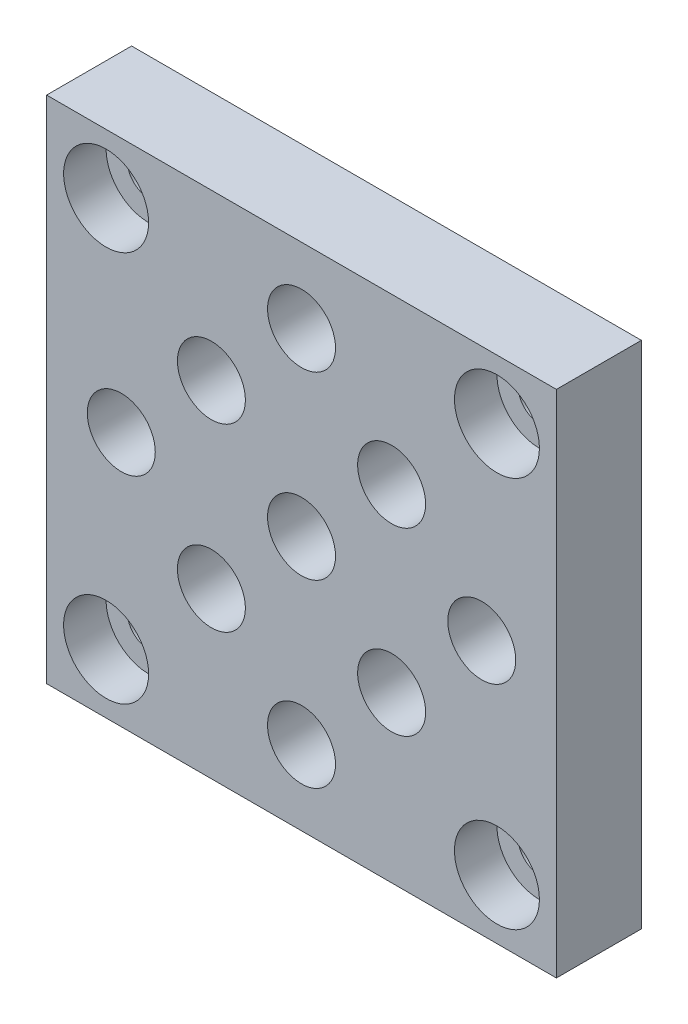
ISO-10303-21;
HEADER;
FILE_DESCRIPTION(('STEP AP214'),'2;1');
FILE_NAME('part.step','',(''),(''),'','','');
FILE_SCHEMA(('AUTOMOTIVE_DESIGN { 1 0 10303 214 1 1 1 1 }'));
ENDSEC;
DATA;
#1=APPLICATION_CONTEXT('core data for automotive mechanical design processes');
#2=APPLICATION_PROTOCOL_DEFINITION('international standard','automotive_design',2000,#1);
#3=PRODUCT_CONTEXT('',#1,'mechanical');
#4=PRODUCT('Part','Part','',(#3));
#5=PRODUCT_RELATED_PRODUCT_CATEGORY('part','',(#4));
#6=PRODUCT_DEFINITION_FORMATION('','',#4);
#7=PRODUCT_DEFINITION_CONTEXT('part definition',#1,'design');
#8=PRODUCT_DEFINITION('design','',#6,#7);
#9=PRODUCT_DEFINITION_SHAPE('','',#8);
#10=(LENGTH_UNIT() NAMED_UNIT(*) SI_UNIT(.MILLI.,.METRE.));
#11=(NAMED_UNIT(*) PLANE_ANGLE_UNIT() SI_UNIT($,.RADIAN.));
#12=(NAMED_UNIT(*) SI_UNIT($,.STERADIAN.) SOLID_ANGLE_UNIT());
#13=UNCERTAINTY_MEASURE_WITH_UNIT(LENGTH_MEASURE(1.E-05),#10,'distance_accuracy_value','');
#14=(GEOMETRIC_REPRESENTATION_CONTEXT(3) GLOBAL_UNCERTAINTY_ASSIGNED_CONTEXT((#13)) GLOBAL_UNIT_ASSIGNED_CONTEXT((#10,
#11,#12)) REPRESENTATION_CONTEXT('',''));
#15=CARTESIAN_POINT('',(0.,0.,0.));
#16=DIRECTION('',(0.,0.,1.));
#17=DIRECTION('',(1.,0.,0.));
#18=AXIS2_PLACEMENT_3D('',#15,#16,#17);
#19=CARTESIAN_POINT('',(0.,60.,10.));
#20=DIRECTION('',(1.,0.,0.));
#21=DIRECTION('',(0.,0.,-1.));
#22=AXIS2_PLACEMENT_3D('',#19,#20,#21);
#23=PLANE('',#22);
#24=DIRECTION('',(0.,-1.,0.));
#25=VECTOR('',#24,1.);
#26=CARTESIAN_POINT('',(0.,60.,0.));
#27=LINE('',#26,#25);
#28=CARTESIAN_POINT('',(0.,60.,0.));
#29=VERTEX_POINT('',#28);
#30=CARTESIAN_POINT('',(0.,0.,0.));
#31=VERTEX_POINT('',#30);
#32=EDGE_CURVE('E117',#29,#31,#27,.T.);
#33=ORIENTED_EDGE('',*,*,#32,.T.);
#34=DIRECTION('',(0.,0.,-1.));
#35=VECTOR('',#34,1.);
#36=CARTESIAN_POINT('',(0.,0.,10.));
#37=LINE('',#36,#35);
#38=CARTESIAN_POINT('',(0.,0.,10.));
#39=VERTEX_POINT('',#38);
#40=EDGE_CURVE('E12',#39,#31,#37,.T.);
#41=ORIENTED_EDGE('',*,*,#40,.F.);
#42=DIRECTION('',(0.,-1.,0.));
#43=VECTOR('',#42,1.);
#44=CARTESIAN_POINT('',(0.,60.,10.));
#45=LINE('',#44,#43);
#46=CARTESIAN_POINT('',(0.,60.,10.));
#47=VERTEX_POINT('',#46);
#48=EDGE_CURVE('E106',#47,#39,#45,.T.);
#49=ORIENTED_EDGE('',*,*,#48,.F.);
#50=DIRECTION('',(0.,0.,-1.));
#51=VECTOR('',#50,1.);
#52=CARTESIAN_POINT('',(0.,60.,10.));
#53=LINE('',#52,#51);
#54=EDGE_CURVE('E111',#47,#29,#53,.T.);
#55=ORIENTED_EDGE('',*,*,#54,.T.);
#56=EDGE_LOOP('',(#33,#41,#49,#55));
#57=FACE_BOUND('',#56,.T.);
#58=ADVANCED_FACE('F54',(#57),#23,.F.);
#59=CARTESIAN_POINT('',(0.,0.,10.));
#60=DIRECTION('',(0.,1.,0.));
#61=DIRECTION('',(0.,0.,1.));
#62=AXIS2_PLACEMENT_3D('',#59,#60,#61);
#63=PLANE('',#62);
#64=DIRECTION('',(1.,0.,0.));
#65=VECTOR('',#64,1.);
#66=CARTESIAN_POINT('',(0.,0.,0.));
#67=LINE('',#66,#65);
#68=CARTESIAN_POINT('',(60.,0.,0.));
#69=VERTEX_POINT('',#68);
#70=EDGE_CURVE('E109',#31,#69,#67,.T.);
#71=ORIENTED_EDGE('',*,*,#70,.T.);
#72=DIRECTION('',(0.,0.,-1.));
#73=VECTOR('',#72,1.);
#74=CARTESIAN_POINT('',(60.,0.,10.));
#75=LINE('',#74,#73);
#76=CARTESIAN_POINT('',(60.,0.,10.));
#77=VERTEX_POINT('',#76);
#78=EDGE_CURVE('E62',#77,#69,#75,.T.);
#79=ORIENTED_EDGE('',*,*,#78,.F.);
#80=DIRECTION('',(1.,0.,0.));
#81=VECTOR('',#80,1.);
#82=CARTESIAN_POINT('',(0.,0.,10.));
#83=LINE('',#82,#81);
#84=EDGE_CURVE('E101',#39,#77,#83,.T.);
#85=ORIENTED_EDGE('',*,*,#84,.F.);
#86=ORIENTED_EDGE('',*,*,#40,.T.);
#87=EDGE_LOOP('',(#71,#79,#85,#86));
#88=FACE_BOUND('',#87,.T.);
#89=ADVANCED_FACE('F108',(#88),#63,.F.);
#90=CARTESIAN_POINT('',(60.,0.,10.));
#91=DIRECTION('',(-1.,0.,0.));
#92=DIRECTION('',(0.,0.,1.));
#93=AXIS2_PLACEMENT_3D('',#90,#91,#92);
#94=PLANE('',#93);
#95=DIRECTION('',(0.,1.,0.));
#96=VECTOR('',#95,1.);
#97=CARTESIAN_POINT('',(60.,0.,0.));
#98=LINE('',#97,#96);
#99=CARTESIAN_POINT('',(60.,60.,0.));
#100=VERTEX_POINT('',#99);
#101=EDGE_CURVE('E86',#69,#100,#98,.T.);
#102=ORIENTED_EDGE('',*,*,#101,.T.);
#103=DIRECTION('',(0.,0.,-1.));
#104=VECTOR('',#103,1.);
#105=CARTESIAN_POINT('',(60.,60.,10.));
#106=LINE('',#105,#104);
#107=CARTESIAN_POINT('',(60.,60.,10.));
#108=VERTEX_POINT('',#107);
#109=EDGE_CURVE('E112',#108,#100,#106,.T.);
#110=ORIENTED_EDGE('',*,*,#109,.F.);
#111=DIRECTION('',(0.,1.,0.));
#112=VECTOR('',#111,1.);
#113=CARTESIAN_POINT('',(60.,0.,10.));
#114=LINE('',#113,#112);
#115=EDGE_CURVE('E102',#77,#108,#114,.T.);
#116=ORIENTED_EDGE('',*,*,#115,.F.);
#117=ORIENTED_EDGE('',*,*,#78,.T.);
#118=EDGE_LOOP('',(#102,#110,#116,#117));
#119=FACE_BOUND('',#118,.T.);
#120=ADVANCED_FACE('F115',(#119),#94,.F.);
#121=CARTESIAN_POINT('',(60.,60.,10.));
#122=DIRECTION('',(0.,-1.,0.));
#123=DIRECTION('',(0.,0.,-1.));
#124=AXIS2_PLACEMENT_3D('',#121,#122,#123);
#125=PLANE('',#124);
#126=DIRECTION('',(-1.,0.,0.));
#127=VECTOR('',#126,1.);
#128=CARTESIAN_POINT('',(60.,60.,0.));
#129=LINE('',#128,#127);
#130=EDGE_CURVE('E94',#100,#29,#129,.T.);
#131=ORIENTED_EDGE('',*,*,#130,.T.);
#132=ORIENTED_EDGE('',*,*,#54,.F.);
#133=DIRECTION('',(-1.,0.,0.));
#134=VECTOR('',#133,1.);
#135=CARTESIAN_POINT('',(60.,60.,10.));
#136=LINE('',#135,#134);
#137=EDGE_CURVE('E72',#108,#47,#136,.T.);
#138=ORIENTED_EDGE('',*,*,#137,.F.);
#139=ORIENTED_EDGE('',*,*,#109,.T.);
#140=EDGE_LOOP('',(#131,#132,#138,#139));
#141=FACE_BOUND('',#140,.T.);
#142=ADVANCED_FACE('F127',(#141),#125,.F.);
#143=CARTESIAN_POINT('',(0.,0.,10.));
#144=DIRECTION('',(0.,0.,1.));
#145=DIRECTION('',(1.,0.,0.));
#146=AXIS2_PLACEMENT_3D('',#143,#144,#145);
#147=PLANE('',#146);
#148=CARTESIAN_POINT('',(30.,51.2132034355964,10.));
#149=DIRECTION('',(0.,0.,1.));
#150=DIRECTION('',(1.,0.,0.));
#151=AXIS2_PLACEMENT_3D('',#148,#149,#150);
#152=CIRCLE('',#151,3.99999999999999);
#153=CARTESIAN_POINT('',(34.,51.2132034355964,10.));
#154=VERTEX_POINT('',#153);
#155=EDGE_CURVE('E181',#154,#154,#152,.T.);
#156=ORIENTED_EDGE('',*,*,#155,.F.);
#157=EDGE_LOOP('',(#156));
#158=FACE_BOUND('',#157,.T.);
#159=CARTESIAN_POINT('',(40.6066017177982,40.6066017177982,10.));
#160=DIRECTION('',(0.,0.,1.));
#161=DIRECTION('',(1.,0.,0.));
#162=AXIS2_PLACEMENT_3D('',#159,#160,#161);
#163=CIRCLE('',#162,4.);
#164=CARTESIAN_POINT('',(44.6066017177982,40.6066017177982,10.));
#165=VERTEX_POINT('',#164);
#166=EDGE_CURVE('E205',#165,#165,#163,.T.);
#167=ORIENTED_EDGE('',*,*,#166,.F.);
#168=EDGE_LOOP('',(#167));
#169=FACE_BOUND('',#168,.T.);
#170=CARTESIAN_POINT('',(51.2132034355964,30.,10.));
#171=DIRECTION('',(0.,0.,1.));
#172=DIRECTION('',(1.,0.,0.));
#173=AXIS2_PLACEMENT_3D('',#170,#171,#172);
#174=CIRCLE('',#173,4.);
#175=CARTESIAN_POINT('',(55.2132034355964,30.,10.));
#176=VERTEX_POINT('',#175);
#177=EDGE_CURVE('E198',#176,#176,#174,.T.);
#178=ORIENTED_EDGE('',*,*,#177,.F.);
#179=EDGE_LOOP('',(#178));
#180=FACE_BOUND('',#179,.T.);
#181=CARTESIAN_POINT('',(40.6066017177982,19.3933982822018,10.));
#182=DIRECTION('',(0.,0.,1.));
#183=DIRECTION('',(1.,0.,0.));
#184=AXIS2_PLACEMENT_3D('',#181,#182,#183);
#185=CIRCLE('',#184,4.);
#186=CARTESIAN_POINT('',(44.6066017177982,19.3933982822018,10.));
#187=VERTEX_POINT('',#186);
#188=EDGE_CURVE('E188',#187,#187,#185,.T.);
#189=ORIENTED_EDGE('',*,*,#188,.F.);
#190=EDGE_LOOP('',(#189));
#191=FACE_BOUND('',#190,.T.);
#192=CARTESIAN_POINT('',(8.78679656440358,30.,10.));
#193=DIRECTION('',(0.,0.,1.));
#194=DIRECTION('',(1.,0.,0.));
#195=AXIS2_PLACEMENT_3D('',#192,#193,#194);
#196=CIRCLE('',#195,4.);
#197=CARTESIAN_POINT('',(12.7867965644036,30.,10.));
#198=VERTEX_POINT('',#197);
#199=EDGE_CURVE('E189',#198,#198,#196,.T.);
#200=ORIENTED_EDGE('',*,*,#199,.F.);
#201=EDGE_LOOP('',(#200));
#202=FACE_BOUND('',#201,.T.);
#203=CARTESIAN_POINT('',(30.,30.,10.));
#204=DIRECTION('',(0.,0.,1.));
#205=DIRECTION('',(1.,0.,0.));
#206=AXIS2_PLACEMENT_3D('',#203,#204,#205);
#207=CIRCLE('',#206,4.);
#208=CARTESIAN_POINT('',(34.,30.,10.));
#209=VERTEX_POINT('',#208);
#210=EDGE_CURVE('E223',#209,#209,#207,.T.);
#211=ORIENTED_EDGE('',*,*,#210,.F.);
#212=EDGE_LOOP('',(#211));
#213=FACE_BOUND('',#212,.T.);
#214=CARTESIAN_POINT('',(19.3933982822018,19.3933982822018,10.));
#215=DIRECTION('',(0.,0.,1.));
#216=DIRECTION('',(1.,0.,0.));
#217=AXIS2_PLACEMENT_3D('',#214,#215,#216);
#218=CIRCLE('',#217,4.);
#219=CARTESIAN_POINT('',(23.3933982822018,19.3933982822018,10.));
#220=VERTEX_POINT('',#219);
#221=EDGE_CURVE('E218',#220,#220,#218,.T.);
#222=ORIENTED_EDGE('',*,*,#221,.F.);
#223=EDGE_LOOP('',(#222));
#224=FACE_BOUND('',#223,.T.);
#225=CARTESIAN_POINT('',(30.,8.78679656440357,10.));
#226=DIRECTION('',(0.,0.,1.));
#227=DIRECTION('',(1.,0.,0.));
#228=AXIS2_PLACEMENT_3D('',#225,#226,#227);
#229=CIRCLE('',#228,4.);
#230=CARTESIAN_POINT('',(34.,8.78679656440357,10.));
#231=VERTEX_POINT('',#230);
#232=EDGE_CURVE('E213',#231,#231,#229,.T.);
#233=ORIENTED_EDGE('',*,*,#232,.F.);
#234=EDGE_LOOP('',(#233));
#235=FACE_BOUND('',#234,.T.);
#236=CARTESIAN_POINT('',(19.3933982822018,40.6066017177982,10.));
#237=DIRECTION('',(0.,0.,1.));
#238=DIRECTION('',(1.,0.,0.));
#239=AXIS2_PLACEMENT_3D('',#236,#237,#238);
#240=CIRCLE('',#239,4.);
#241=CARTESIAN_POINT('',(23.3933982822018,40.6066017177982,10.));
#242=VERTEX_POINT('',#241);
#243=EDGE_CURVE('E180',#242,#242,#240,.T.);
#244=ORIENTED_EDGE('',*,*,#243,.F.);
#245=EDGE_LOOP('',(#244));
#246=FACE_BOUND('',#245,.T.);
#247=CARTESIAN_POINT('',(53.,53.,10.));
#248=DIRECTION('',(0.,0.,1.));
#249=DIRECTION('',(1.,0.,0.));
#250=AXIS2_PLACEMENT_3D('',#247,#248,#249);
#251=CIRCLE('',#250,5.00000000000001);
#252=CARTESIAN_POINT('',(58.,53.,10.));
#253=VERTEX_POINT('',#252);
#254=EDGE_CURVE('E144',#253,#253,#251,.T.);
#255=ORIENTED_EDGE('',*,*,#254,.F.);
#256=EDGE_LOOP('',(#255));
#257=FACE_BOUND('',#256,.T.);
#258=CARTESIAN_POINT('',(7.,7.,10.));
#259=DIRECTION('',(0.,0.,1.));
#260=DIRECTION('',(1.,0.,0.));
#261=AXIS2_PLACEMENT_3D('',#258,#259,#260);
#262=CIRCLE('',#261,5.);
#263=CARTESIAN_POINT('',(12.,7.,10.));
#264=VERTEX_POINT('',#263);
#265=EDGE_CURVE('E139',#264,#264,#262,.T.);
#266=ORIENTED_EDGE('',*,*,#265,.F.);
#267=EDGE_LOOP('',(#266));
#268=FACE_BOUND('',#267,.T.);
#269=CARTESIAN_POINT('',(53.,7.,10.));
#270=DIRECTION('',(0.,0.,1.));
#271=DIRECTION('',(1.,0.,0.));
#272=AXIS2_PLACEMENT_3D('',#269,#270,#271);
#273=CIRCLE('',#272,5.);
#274=CARTESIAN_POINT('',(58.,7.,10.));
#275=VERTEX_POINT('',#274);
#276=EDGE_CURVE('E147',#275,#275,#273,.T.);
#277=ORIENTED_EDGE('',*,*,#276,.F.);
#278=EDGE_LOOP('',(#277));
#279=FACE_BOUND('',#278,.T.);
#280=CARTESIAN_POINT('',(7.,53.,10.));
#281=DIRECTION('',(0.,0.,1.));
#282=DIRECTION('',(1.,0.,0.));
#283=AXIS2_PLACEMENT_3D('',#280,#281,#282);
#284=CIRCLE('',#283,5.);
#285=CARTESIAN_POINT('',(12.,53.,10.));
#286=VERTEX_POINT('',#285);
#287=EDGE_CURVE('E135',#286,#286,#284,.T.);
#288=ORIENTED_EDGE('',*,*,#287,.F.);
#289=EDGE_LOOP('',(#288));
#290=FACE_BOUND('',#289,.T.);
#291=ORIENTED_EDGE('',*,*,#48,.T.);
#292=ORIENTED_EDGE('',*,*,#84,.T.);
#293=ORIENTED_EDGE('',*,*,#115,.T.);
#294=ORIENTED_EDGE('',*,*,#137,.T.);
#295=EDGE_LOOP('',(#291,#292,#293,#294));
#296=FACE_BOUND('',#295,.T.);
#297=ADVANCED_FACE('F105',(#158,#169,#180,#191,#202,#213,#224,#235,#246,#257,#268,#279,#290,
#296),#147,.T.);
#298=CARTESIAN_POINT('',(0.,0.,0.));
#299=DIRECTION('',(0.,0.,1.));
#300=DIRECTION('',(1.,0.,0.));
#301=AXIS2_PLACEMENT_3D('',#298,#299,#300);
#302=PLANE('',#301);
#303=CARTESIAN_POINT('',(30.,51.2132034355964,0.));
#304=DIRECTION('',(0.,0.,1.));
#305=DIRECTION('',(1.,0.,0.));
#306=AXIS2_PLACEMENT_3D('',#303,#304,#305);
#307=CIRCLE('',#306,3.99999999999999);
#308=CARTESIAN_POINT('',(34.,51.2132034355964,0.));
#309=VERTEX_POINT('',#308);
#310=EDGE_CURVE('E202',#309,#309,#307,.T.);
#311=ORIENTED_EDGE('',*,*,#310,.T.);
#312=EDGE_LOOP('',(#311));
#313=FACE_BOUND('',#312,.T.);
#314=CARTESIAN_POINT('',(40.6066017177982,40.6066017177982,0.));
#315=DIRECTION('',(0.,0.,1.));
#316=DIRECTION('',(1.,0.,0.));
#317=AXIS2_PLACEMENT_3D('',#314,#315,#316);
#318=CIRCLE('',#317,4.);
#319=CARTESIAN_POINT('',(44.6066017177982,40.6066017177982,0.));
#320=VERTEX_POINT('',#319);
#321=EDGE_CURVE('E200',#320,#320,#318,.T.);
#322=ORIENTED_EDGE('',*,*,#321,.T.);
#323=EDGE_LOOP('',(#322));
#324=FACE_BOUND('',#323,.T.);
#325=CARTESIAN_POINT('',(51.2132034355964,30.,0.));
#326=DIRECTION('',(0.,0.,1.));
#327=DIRECTION('',(1.,0.,0.));
#328=AXIS2_PLACEMENT_3D('',#325,#326,#327);
#329=CIRCLE('',#328,4.);
#330=CARTESIAN_POINT('',(55.2132034355964,30.,0.));
#331=VERTEX_POINT('',#330);
#332=EDGE_CURVE('E194',#331,#331,#329,.T.);
#333=ORIENTED_EDGE('',*,*,#332,.T.);
#334=EDGE_LOOP('',(#333));
#335=FACE_BOUND('',#334,.T.);
#336=CARTESIAN_POINT('',(40.6066017177982,19.3933982822018,0.));
#337=DIRECTION('',(0.,0.,1.));
#338=DIRECTION('',(1.,0.,0.));
#339=AXIS2_PLACEMENT_3D('',#336,#337,#338);
#340=CIRCLE('',#339,4.);
#341=CARTESIAN_POINT('',(44.6066017177982,19.3933982822018,0.));
#342=VERTEX_POINT('',#341);
#343=EDGE_CURVE('E186',#342,#342,#340,.T.);
#344=ORIENTED_EDGE('',*,*,#343,.T.);
#345=EDGE_LOOP('',(#344));
#346=FACE_BOUND('',#345,.T.);
#347=CARTESIAN_POINT('',(8.78679656440358,30.,0.));
#348=DIRECTION('',(0.,0.,1.));
#349=DIRECTION('',(1.,0.,0.));
#350=AXIS2_PLACEMENT_3D('',#347,#348,#349);
#351=CIRCLE('',#350,4.);
#352=CARTESIAN_POINT('',(12.7867965644036,30.,0.));
#353=VERTEX_POINT('',#352);
#354=EDGE_CURVE('E227',#353,#353,#351,.T.);
#355=ORIENTED_EDGE('',*,*,#354,.T.);
#356=EDGE_LOOP('',(#355));
#357=FACE_BOUND('',#356,.T.);
#358=CARTESIAN_POINT('',(30.,30.,0.));
#359=DIRECTION('',(0.,0.,1.));
#360=DIRECTION('',(1.,0.,0.));
#361=AXIS2_PLACEMENT_3D('',#358,#359,#360);
#362=CIRCLE('',#361,4.);
#363=CARTESIAN_POINT('',(34.,30.,0.));
#364=VERTEX_POINT('',#363);
#365=EDGE_CURVE('E225',#364,#364,#362,.T.);
#366=ORIENTED_EDGE('',*,*,#365,.T.);
#367=EDGE_LOOP('',(#366));
#368=FACE_BOUND('',#367,.T.);
#369=CARTESIAN_POINT('',(19.3933982822018,19.3933982822018,0.));
#370=DIRECTION('',(0.,0.,1.));
#371=DIRECTION('',(1.,0.,0.));
#372=AXIS2_PLACEMENT_3D('',#369,#370,#371);
#373=CIRCLE('',#372,4.);
#374=CARTESIAN_POINT('',(23.3933982822018,19.3933982822018,0.));
#375=VERTEX_POINT('',#374);
#376=EDGE_CURVE('E216',#375,#375,#373,.T.);
#377=ORIENTED_EDGE('',*,*,#376,.T.);
#378=EDGE_LOOP('',(#377));
#379=FACE_BOUND('',#378,.T.);
#380=CARTESIAN_POINT('',(30.,8.78679656440357,0.));
#381=DIRECTION('',(0.,0.,1.));
#382=DIRECTION('',(1.,0.,0.));
#383=AXIS2_PLACEMENT_3D('',#380,#381,#382);
#384=CIRCLE('',#383,4.);
#385=CARTESIAN_POINT('',(34.,8.78679656440357,0.));
#386=VERTEX_POINT('',#385);
#387=EDGE_CURVE('E209',#386,#386,#384,.T.);
#388=ORIENTED_EDGE('',*,*,#387,.T.);
#389=EDGE_LOOP('',(#388));
#390=FACE_BOUND('',#389,.T.);
#391=CARTESIAN_POINT('',(19.3933982822018,40.6066017177982,0.));
#392=DIRECTION('',(0.,0.,1.));
#393=DIRECTION('',(1.,0.,0.));
#394=AXIS2_PLACEMENT_3D('',#391,#392,#393);
#395=CIRCLE('',#394,4.);
#396=CARTESIAN_POINT('',(23.3933982822018,40.6066017177982,0.));
#397=VERTEX_POINT('',#396);
#398=EDGE_CURVE('E177',#397,#397,#395,.T.);
#399=ORIENTED_EDGE('',*,*,#398,.T.);
#400=EDGE_LOOP('',(#399));
#401=FACE_BOUND('',#400,.T.);
#402=CARTESIAN_POINT('',(53.,53.,0.));
#403=DIRECTION('',(0.,0.,1.));
#404=DIRECTION('',(1.,0.,0.));
#405=AXIS2_PLACEMENT_3D('',#402,#403,#404);
#406=CIRCLE('',#405,2.5);
#407=CARTESIAN_POINT('',(55.5,53.,0.));
#408=VERTEX_POINT('',#407);
#409=EDGE_CURVE('E157',#408,#408,#406,.T.);
#410=ORIENTED_EDGE('',*,*,#409,.T.);
#411=EDGE_LOOP('',(#410));
#412=FACE_BOUND('',#411,.T.);
#413=CARTESIAN_POINT('',(7.,7.,0.));
#414=DIRECTION('',(0.,0.,1.));
#415=DIRECTION('',(1.,0.,0.));
#416=AXIS2_PLACEMENT_3D('',#413,#414,#415);
#417=CIRCLE('',#416,2.5);
#418=CARTESIAN_POINT('',(9.5,7.,0.));
#419=VERTEX_POINT('',#418);
#420=EDGE_CURVE('E164',#419,#419,#417,.T.);
#421=ORIENTED_EDGE('',*,*,#420,.T.);
#422=EDGE_LOOP('',(#421));
#423=FACE_BOUND('',#422,.T.);
#424=CARTESIAN_POINT('',(53.,7.,0.));
#425=DIRECTION('',(0.,0.,1.));
#426=DIRECTION('',(1.,0.,0.));
#427=AXIS2_PLACEMENT_3D('',#424,#425,#426);
#428=CIRCLE('',#427,2.49999999999999);
#429=CARTESIAN_POINT('',(55.5,7.,0.));
#430=VERTEX_POINT('',#429);
#431=EDGE_CURVE('E167',#430,#430,#428,.T.);
#432=ORIENTED_EDGE('',*,*,#431,.T.);
#433=EDGE_LOOP('',(#432));
#434=FACE_BOUND('',#433,.T.);
#435=CARTESIAN_POINT('',(7.,53.,0.));
#436=DIRECTION('',(0.,0.,1.));
#437=DIRECTION('',(1.,0.,0.));
#438=AXIS2_PLACEMENT_3D('',#435,#436,#437);
#439=CIRCLE('',#438,2.5);
#440=CARTESIAN_POINT('',(9.5,53.,0.));
#441=VERTEX_POINT('',#440);
#442=EDGE_CURVE('E153',#441,#441,#439,.T.);
#443=ORIENTED_EDGE('',*,*,#442,.T.);
#444=EDGE_LOOP('',(#443));
#445=FACE_BOUND('',#444,.T.);
#446=ORIENTED_EDGE('',*,*,#32,.F.);
#447=ORIENTED_EDGE('',*,*,#130,.F.);
#448=ORIENTED_EDGE('',*,*,#101,.F.);
#449=ORIENTED_EDGE('',*,*,#70,.F.);
#450=EDGE_LOOP('',(#446,#447,#448,#449));
#451=FACE_BOUND('',#450,.T.);
#452=ADVANCED_FACE('F129',(#313,#324,#335,#346,#357,#368,#379,#390,#401,#412,#423,#434,#445,
#451),#302,.F.);
#453=CARTESIAN_POINT('',(7.,53.,5.));
#454=DIRECTION('',(0.,0.,1.));
#455=DIRECTION('',(1.,0.,0.));
#456=AXIS2_PLACEMENT_3D('',#453,#454,#455);
#457=CYLINDRICAL_SURFACE('',#456,5.);
#458=CARTESIAN_POINT('',(7.,53.,5.));
#459=DIRECTION('',(0.,0.,1.));
#460=DIRECTION('',(1.,0.,0.));
#461=AXIS2_PLACEMENT_3D('',#458,#459,#460);
#462=CIRCLE('',#461,5.);
#463=CARTESIAN_POINT('',(12.,53.,5.));
#464=VERTEX_POINT('',#463);
#465=EDGE_CURVE('E121',#464,#464,#462,.T.);
#466=ORIENTED_EDGE('',*,*,#465,.F.);
#467=EDGE_LOOP('',(#466));
#468=FACE_BOUND('',#467,.T.);
#469=ORIENTED_EDGE('',*,*,#287,.T.);
#470=EDGE_LOOP('',(#469));
#471=FACE_BOUND('',#470,.T.);
#472=ADVANCED_FACE('F258',(#468,#471),#457,.F.);
#473=CARTESIAN_POINT('',(7.,53.,5.));
#474=DIRECTION('',(0.,0.,1.));
#475=DIRECTION('',(1.,0.,0.));
#476=AXIS2_PLACEMENT_3D('',#473,#474,#475);
#477=PLANE('',#476);
#478=CARTESIAN_POINT('',(7.,53.,5.));
#479=DIRECTION('',(0.,0.,1.));
#480=DIRECTION('',(1.,0.,0.));
#481=AXIS2_PLACEMENT_3D('',#478,#479,#480);
#482=CIRCLE('',#481,2.5);
#483=CARTESIAN_POINT('',(9.5,53.,5.));
#484=VERTEX_POINT('',#483);
#485=EDGE_CURVE('E156',#484,#484,#482,.T.);
#486=ORIENTED_EDGE('',*,*,#485,.F.);
#487=EDGE_LOOP('',(#486));
#488=FACE_BOUND('',#487,.T.);
#489=ORIENTED_EDGE('',*,*,#465,.T.);
#490=EDGE_LOOP('',(#489));
#491=FACE_BOUND('',#490,.T.);
#492=ADVANCED_FACE('F256',(#488,#491),#477,.T.);
#493=CARTESIAN_POINT('',(53.,7.,5.));
#494=DIRECTION('',(0.,0.,1.));
#495=DIRECTION('',(1.,0.,0.));
#496=AXIS2_PLACEMENT_3D('',#493,#494,#495);
#497=CYLINDRICAL_SURFACE('',#496,5.);
#498=CARTESIAN_POINT('',(53.,7.,5.));
#499=DIRECTION('',(0.,0.,1.));
#500=DIRECTION('',(1.,0.,0.));
#501=AXIS2_PLACEMENT_3D('',#498,#499,#500);
#502=CIRCLE('',#501,5.);
#503=CARTESIAN_POINT('',(58.,7.,5.));
#504=VERTEX_POINT('',#503);
#505=EDGE_CURVE('E142',#504,#504,#502,.T.);
#506=ORIENTED_EDGE('',*,*,#505,.F.);
#507=EDGE_LOOP('',(#506));
#508=FACE_BOUND('',#507,.T.);
#509=ORIENTED_EDGE('',*,*,#276,.T.);
#510=EDGE_LOOP('',(#509));
#511=FACE_BOUND('',#510,.T.);
#512=ADVANCED_FACE('F264',(#508,#511),#497,.F.);
#513=CARTESIAN_POINT('',(53.,7.,5.));
#514=DIRECTION('',(0.,0.,1.));
#515=DIRECTION('',(1.,0.,0.));
#516=AXIS2_PLACEMENT_3D('',#513,#514,#515);
#517=PLANE('',#516);
#518=CARTESIAN_POINT('',(53.,7.,5.));
#519=DIRECTION('',(0.,0.,1.));
#520=DIRECTION('',(1.,0.,0.));
#521=AXIS2_PLACEMENT_3D('',#518,#519,#520);
#522=CIRCLE('',#521,2.49999999999999);
#523=CARTESIAN_POINT('',(55.5,7.,5.));
#524=VERTEX_POINT('',#523);
#525=EDGE_CURVE('E173',#524,#524,#522,.T.);
#526=ORIENTED_EDGE('',*,*,#525,.F.);
#527=EDGE_LOOP('',(#526));
#528=FACE_BOUND('',#527,.T.);
#529=ORIENTED_EDGE('',*,*,#505,.T.);
#530=EDGE_LOOP('',(#529));
#531=FACE_BOUND('',#530,.T.);
#532=ADVANCED_FACE('F312',(#528,#531),#517,.T.);
#533=CARTESIAN_POINT('',(7.,7.,5.));
#534=DIRECTION('',(0.,0.,1.));
#535=DIRECTION('',(1.,0.,0.));
#536=AXIS2_PLACEMENT_3D('',#533,#534,#535);
#537=CYLINDRICAL_SURFACE('',#536,5.);
#538=CARTESIAN_POINT('',(7.,7.,5.));
#539=DIRECTION('',(0.,0.,1.));
#540=DIRECTION('',(1.,0.,0.));
#541=AXIS2_PLACEMENT_3D('',#538,#539,#540);
#542=CIRCLE('',#541,5.);
#543=CARTESIAN_POINT('',(12.,7.,5.));
#544=VERTEX_POINT('',#543);
#545=EDGE_CURVE('E143',#544,#544,#542,.T.);
#546=ORIENTED_EDGE('',*,*,#545,.F.);
#547=EDGE_LOOP('',(#546));
#548=FACE_BOUND('',#547,.T.);
#549=ORIENTED_EDGE('',*,*,#265,.T.);
#550=EDGE_LOOP('',(#549));
#551=FACE_BOUND('',#550,.T.);
#552=ADVANCED_FACE('F324',(#548,#551),#537,.F.);
#553=CARTESIAN_POINT('',(7.,7.,5.));
#554=DIRECTION('',(0.,0.,1.));
#555=DIRECTION('',(1.,0.,0.));
#556=AXIS2_PLACEMENT_3D('',#553,#554,#555);
#557=PLANE('',#556);
#558=CARTESIAN_POINT('',(7.,7.,5.));
#559=DIRECTION('',(0.,0.,1.));
#560=DIRECTION('',(1.,0.,0.));
#561=AXIS2_PLACEMENT_3D('',#558,#559,#560);
#562=CIRCLE('',#561,2.5);
#563=CARTESIAN_POINT('',(9.5,7.,5.));
#564=VERTEX_POINT('',#563);
#565=EDGE_CURVE('E165',#564,#564,#562,.T.);
#566=ORIENTED_EDGE('',*,*,#565,.F.);
#567=EDGE_LOOP('',(#566));
#568=FACE_BOUND('',#567,.T.);
#569=ORIENTED_EDGE('',*,*,#545,.T.);
#570=EDGE_LOOP('',(#569));
#571=FACE_BOUND('',#570,.T.);
#572=ADVANCED_FACE('F333',(#568,#571),#557,.T.);
#573=CARTESIAN_POINT('',(53.,53.,5.));
#574=DIRECTION('',(0.,0.,1.));
#575=DIRECTION('',(1.,0.,0.));
#576=AXIS2_PLACEMENT_3D('',#573,#574,#575);
#577=CYLINDRICAL_SURFACE('',#576,5.00000000000001);
#578=CARTESIAN_POINT('',(53.,53.,5.));
#579=DIRECTION('',(0.,0.,1.));
#580=DIRECTION('',(1.,0.,0.));
#581=AXIS2_PLACEMENT_3D('',#578,#579,#580);
#582=CIRCLE('',#581,5.00000000000001);
#583=CARTESIAN_POINT('',(58.,53.,5.));
#584=VERTEX_POINT('',#583);
#585=EDGE_CURVE('E134',#584,#584,#582,.T.);
#586=ORIENTED_EDGE('',*,*,#585,.F.);
#587=EDGE_LOOP('',(#586));
#588=FACE_BOUND('',#587,.T.);
#589=ORIENTED_EDGE('',*,*,#254,.T.);
#590=EDGE_LOOP('',(#589));
#591=FACE_BOUND('',#590,.T.);
#592=ADVANCED_FACE('F343',(#588,#591),#577,.F.);
#593=CARTESIAN_POINT('',(53.,53.,5.));
#594=DIRECTION('',(0.,0.,1.));
#595=DIRECTION('',(1.,0.,0.));
#596=AXIS2_PLACEMENT_3D('',#593,#594,#595);
#597=PLANE('',#596);
#598=CARTESIAN_POINT('',(53.,53.,5.));
#599=DIRECTION('',(0.,0.,1.));
#600=DIRECTION('',(1.,0.,0.));
#601=AXIS2_PLACEMENT_3D('',#598,#599,#600);
#602=CIRCLE('',#601,2.5);
#603=CARTESIAN_POINT('',(55.5,53.,5.));
#604=VERTEX_POINT('',#603);
#605=EDGE_CURVE('E166',#604,#604,#602,.T.);
#606=ORIENTED_EDGE('',*,*,#605,.F.);
#607=EDGE_LOOP('',(#606));
#608=FACE_BOUND('',#607,.T.);
#609=ORIENTED_EDGE('',*,*,#585,.T.);
#610=EDGE_LOOP('',(#609));
#611=FACE_BOUND('',#610,.T.);
#612=ADVANCED_FACE('F353',(#608,#611),#597,.T.);
#613=CARTESIAN_POINT('',(7.,53.,0.));
#614=DIRECTION('',(0.,0.,1.));
#615=DIRECTION('',(1.,0.,0.));
#616=AXIS2_PLACEMENT_3D('',#613,#614,#615);
#617=CYLINDRICAL_SURFACE('',#616,2.5);
#618=ORIENTED_EDGE('',*,*,#442,.F.);
#619=EDGE_LOOP('',(#618));
#620=FACE_BOUND('',#619,.T.);
#621=ORIENTED_EDGE('',*,*,#485,.T.);
#622=EDGE_LOOP('',(#621));
#623=FACE_BOUND('',#622,.T.);
#624=ADVANCED_FACE('F361',(#620,#623),#617,.F.);
#625=CARTESIAN_POINT('',(53.,7.,0.));
#626=DIRECTION('',(0.,0.,1.));
#627=DIRECTION('',(1.,0.,0.));
#628=AXIS2_PLACEMENT_3D('',#625,#626,#627);
#629=CYLINDRICAL_SURFACE('',#628,2.49999999999999);
#630=ORIENTED_EDGE('',*,*,#431,.F.);
#631=EDGE_LOOP('',(#630));
#632=FACE_BOUND('',#631,.T.);
#633=ORIENTED_EDGE('',*,*,#525,.T.);
#634=EDGE_LOOP('',(#633));
#635=FACE_BOUND('',#634,.T.);
#636=ADVANCED_FACE('F373',(#632,#635),#629,.F.);
#637=CARTESIAN_POINT('',(7.,7.,0.));
#638=DIRECTION('',(0.,0.,1.));
#639=DIRECTION('',(1.,0.,0.));
#640=AXIS2_PLACEMENT_3D('',#637,#638,#639);
#641=CYLINDRICAL_SURFACE('',#640,2.5);
#642=ORIENTED_EDGE('',*,*,#420,.F.);
#643=EDGE_LOOP('',(#642));
#644=FACE_BOUND('',#643,.T.);
#645=ORIENTED_EDGE('',*,*,#565,.T.);
#646=EDGE_LOOP('',(#645));
#647=FACE_BOUND('',#646,.T.);
#648=ADVANCED_FACE('F382',(#644,#647),#641,.F.);
#649=CARTESIAN_POINT('',(53.,53.,0.));
#650=DIRECTION('',(0.,0.,1.));
#651=DIRECTION('',(1.,0.,0.));
#652=AXIS2_PLACEMENT_3D('',#649,#650,#651);
#653=CYLINDRICAL_SURFACE('',#652,2.5);
#654=ORIENTED_EDGE('',*,*,#409,.F.);
#655=EDGE_LOOP('',(#654));
#656=FACE_BOUND('',#655,.T.);
#657=ORIENTED_EDGE('',*,*,#605,.T.);
#658=EDGE_LOOP('',(#657));
#659=FACE_BOUND('',#658,.T.);
#660=ADVANCED_FACE('F392',(#656,#659),#653,.F.);
#661=CARTESIAN_POINT('',(19.3933982822018,40.6066017177982,0.));
#662=DIRECTION('',(0.,0.,1.));
#663=DIRECTION('',(1.,0.,0.));
#664=AXIS2_PLACEMENT_3D('',#661,#662,#663);
#665=CYLINDRICAL_SURFACE('',#664,4.);
#666=ORIENTED_EDGE('',*,*,#398,.F.);
#667=EDGE_LOOP('',(#666));
#668=FACE_BOUND('',#667,.T.);
#669=ORIENTED_EDGE('',*,*,#243,.T.);
#670=EDGE_LOOP('',(#669));
#671=FACE_BOUND('',#670,.T.);
#672=ADVANCED_FACE('F401',(#668,#671),#665,.F.);
#673=CARTESIAN_POINT('',(30.,8.78679656440357,0.));
#674=DIRECTION('',(0.,0.,1.));
#675=DIRECTION('',(1.,0.,0.));
#676=AXIS2_PLACEMENT_3D('',#673,#674,#675);
#677=CYLINDRICAL_SURFACE('',#676,4.);
#678=ORIENTED_EDGE('',*,*,#232,.T.);
#679=EDGE_LOOP('',(#678));
#680=FACE_BOUND('',#679,.T.);
#681=ORIENTED_EDGE('',*,*,#387,.F.);
#682=EDGE_LOOP('',(#681));
#683=FACE_BOUND('',#682,.T.);
#684=ADVANCED_FACE('F412',(#680,#683),#677,.F.);
#685=CARTESIAN_POINT('',(19.3933982822018,19.3933982822018,0.));
#686=DIRECTION('',(0.,0.,1.));
#687=DIRECTION('',(1.,0.,0.));
#688=AXIS2_PLACEMENT_3D('',#685,#686,#687);
#689=CYLINDRICAL_SURFACE('',#688,4.);
#690=ORIENTED_EDGE('',*,*,#376,.F.);
#691=EDGE_LOOP('',(#690));
#692=FACE_BOUND('',#691,.T.);
#693=ORIENTED_EDGE('',*,*,#221,.T.);
#694=EDGE_LOOP('',(#693));
#695=FACE_BOUND('',#694,.T.);
#696=ADVANCED_FACE('F425',(#692,#695),#689,.F.);
#697=CARTESIAN_POINT('',(30.,30.,0.));
#698=DIRECTION('',(0.,0.,1.));
#699=DIRECTION('',(1.,0.,0.));
#700=AXIS2_PLACEMENT_3D('',#697,#698,#699);
#701=CYLINDRICAL_SURFACE('',#700,4.);
#702=ORIENTED_EDGE('',*,*,#365,.F.);
#703=EDGE_LOOP('',(#702));
#704=FACE_BOUND('',#703,.T.);
#705=ORIENTED_EDGE('',*,*,#210,.T.);
#706=EDGE_LOOP('',(#705));
#707=FACE_BOUND('',#706,.T.);
#708=ADVANCED_FACE('F435',(#704,#707),#701,.F.);
#709=CARTESIAN_POINT('',(8.78679656440358,30.,0.));
#710=DIRECTION('',(0.,0.,1.));
#711=DIRECTION('',(1.,0.,0.));
#712=AXIS2_PLACEMENT_3D('',#709,#710,#711);
#713=CYLINDRICAL_SURFACE('',#712,4.);
#714=ORIENTED_EDGE('',*,*,#354,.F.);
#715=EDGE_LOOP('',(#714));
#716=FACE_BOUND('',#715,.T.);
#717=ORIENTED_EDGE('',*,*,#199,.T.);
#718=EDGE_LOOP('',(#717));
#719=FACE_BOUND('',#718,.T.);
#720=ADVANCED_FACE('F233',(#716,#719),#713,.F.);
#721=CARTESIAN_POINT('',(40.6066017177982,19.3933982822018,0.));
#722=DIRECTION('',(0.,0.,1.));
#723=DIRECTION('',(1.,0.,0.));
#724=AXIS2_PLACEMENT_3D('',#721,#722,#723);
#725=CYLINDRICAL_SURFACE('',#724,4.);
#726=ORIENTED_EDGE('',*,*,#343,.F.);
#727=EDGE_LOOP('',(#726));
#728=FACE_BOUND('',#727,.T.);
#729=ORIENTED_EDGE('',*,*,#188,.T.);
#730=EDGE_LOOP('',(#729));
#731=FACE_BOUND('',#730,.T.);
#732=ADVANCED_FACE('F451',(#728,#731),#725,.F.);
#733=CARTESIAN_POINT('',(51.2132034355964,30.,0.));
#734=DIRECTION('',(0.,0.,1.));
#735=DIRECTION('',(1.,0.,0.));
#736=AXIS2_PLACEMENT_3D('',#733,#734,#735);
#737=CYLINDRICAL_SURFACE('',#736,4.);
#738=ORIENTED_EDGE('',*,*,#332,.F.);
#739=EDGE_LOOP('',(#738));
#740=FACE_BOUND('',#739,.T.);
#741=ORIENTED_EDGE('',*,*,#177,.T.);
#742=EDGE_LOOP('',(#741));
#743=FACE_BOUND('',#742,.T.);
#744=ADVANCED_FACE('F461',(#740,#743),#737,.F.);
#745=CARTESIAN_POINT('',(40.6066017177982,40.6066017177982,0.));
#746=DIRECTION('',(0.,0.,1.));
#747=DIRECTION('',(1.,0.,0.));
#748=AXIS2_PLACEMENT_3D('',#745,#746,#747);
#749=CYLINDRICAL_SURFACE('',#748,4.);
#750=ORIENTED_EDGE('',*,*,#321,.F.);
#751=EDGE_LOOP('',(#750));
#752=FACE_BOUND('',#751,.T.);
#753=ORIENTED_EDGE('',*,*,#166,.T.);
#754=EDGE_LOOP('',(#753));
#755=FACE_BOUND('',#754,.T.);
#756=ADVANCED_FACE('F473',(#752,#755),#749,.F.);
#757=CARTESIAN_POINT('',(30.,51.2132034355964,0.));
#758=DIRECTION('',(0.,0.,1.));
#759=DIRECTION('',(1.,0.,0.));
#760=AXIS2_PLACEMENT_3D('',#757,#758,#759);
#761=CYLINDRICAL_SURFACE('',#760,3.99999999999999);
#762=ORIENTED_EDGE('',*,*,#310,.F.);
#763=EDGE_LOOP('',(#762));
#764=FACE_BOUND('',#763,.T.);
#765=ORIENTED_EDGE('',*,*,#155,.T.);
#766=EDGE_LOOP('',(#765));
#767=FACE_BOUND('',#766,.T.);
#768=ADVANCED_FACE('F481',(#764,#767),#761,.F.);
#769=CLOSED_SHELL('',(#58,#89,#120,#142,#297,#452,#472,#492,#512,#532,#552,#572,#592,#612,#624,
#636,#648,#660,#672,#684,#696,#708,#720,#732,#744,#756,#768));
#770=MANIFOLD_SOLID_BREP('B2',#769);
#771=ADVANCED_BREP_SHAPE_REPRESENTATION('',(#18,#770),#14);
#772=SHAPE_DEFINITION_REPRESENTATION(#9,#771);
ENDSEC;
END-ISO-10303-21;
